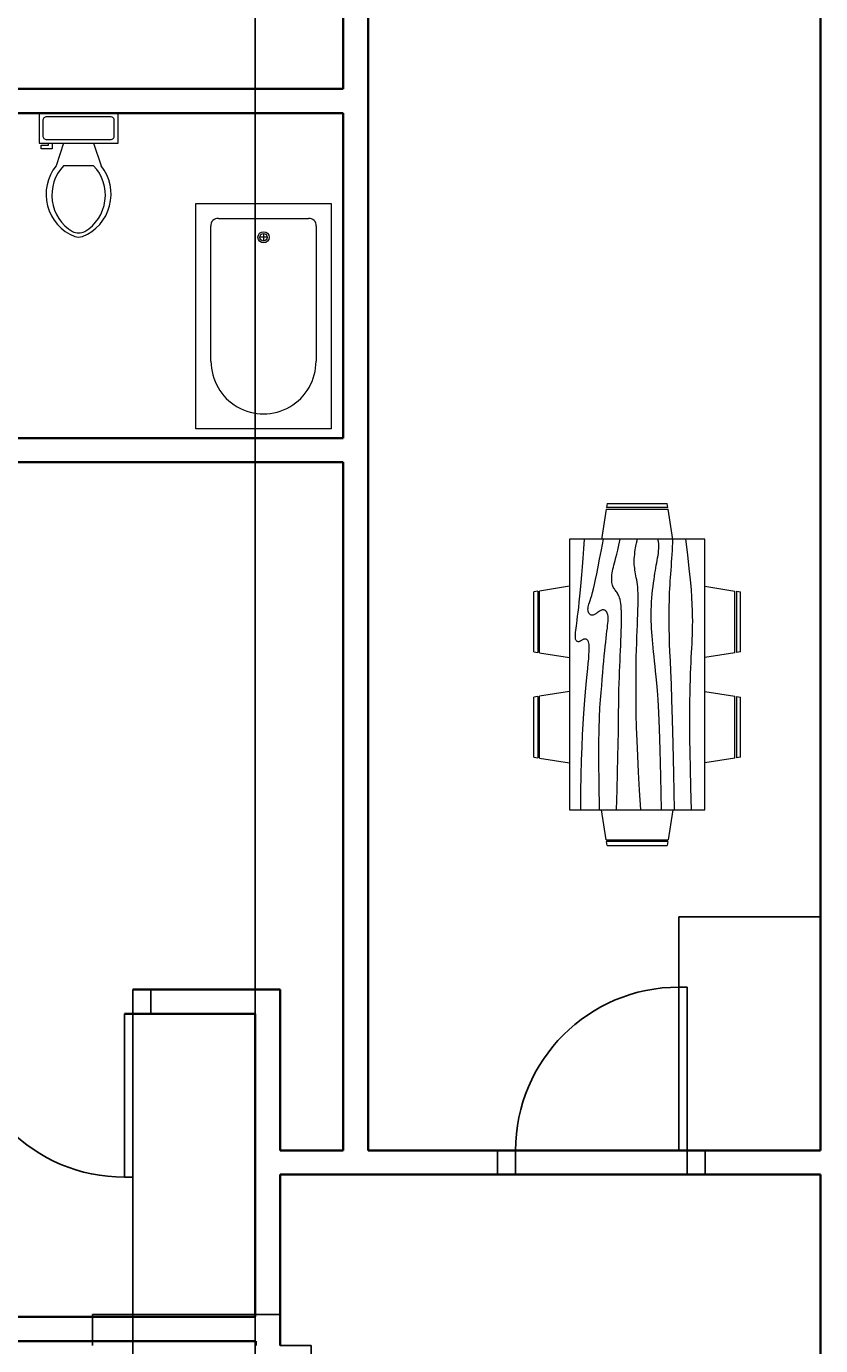
# Model space of a CAD drawing. Units: millimetres. Extents: x 31 to 27050, y -916 to 32407.
# Tile 5 of 7: x 7965 to 13341, y 16782 to 25704. Entities that reach past the tile are written whole.
import ezdxf

# ---------------------------------------------------------------- set-up
doc = ezdxf.new("R2010")
doc.units = ezdxf.units.MM
for name, color, linetype, lineweight in [('A-ANNO-DIMS', 2, 'Continuous', 18), ('A-DOOR', 3, 'Continuous', 25), ('A-FLOR-FIXT', 9, 'Continuous', 18), ('A-FURN', 8, 'Continuous', 13), ('A-WALL', 7, 'Continuous', 35)]:
    doc.layers.add(name, color=color, linetype=linetype, lineweight=lineweight)
doc.styles.get("Standard").update_dxf_attribs({"font": 'arial.ttf'})
doc.dimstyles.get("Standard").update_dxf_attribs({"dimtxt": 0.18, "dimasz": 0.18, "dimexe": 0.18, "dimexo": 0.0625, "dimgap": 0.09, "dimtad": 0, "dimtih": 1, "dimtoh": 1, "dimdec": 4, "dimzin": 0, "dimdsep": 46, "dimtxsty": 'Standard', "dimcen": 0.09, "dimadec": 0, "dimazin": 0, "dimtfac": 1, "dimtdec": 4, "dimtofl": 0, "dimtmove": 0, "dimatfit": 3, "dimfxl": 1, "dimtolj": 1, "dimtzin": 0, "dimarcsym": 0})

# ---------------------------------------------------------------- blocks, each defined once
blk = doc.blocks.new('Dining Set - 36 x 72 in.')
for p, q in [((-22.23430000000002, 26.00059), (-23.48470000000003, 17.99762)), ((-22.23040000000003, 26), (-5.760800000000017, 26)), ((-22, 27.5), (-22.15620000000001, 26.50042)), ((-5.841600000000028, 26.5), (-22.15340000000003, 26.5)), ((-22, 27.5), (-6, 27.5)), ((-5.843700000000012, 26.49966), (-6, 27.5)), ((-4.515199999999992, 17.99762), (-5.765500000000031, 25.99926)), ((5.765699999999981, 26.00059), (4.515299999999967, 17.99762)), ((5.769599999999968, 26), (22.23919999999998, 26)), ((6, 27.5), (5.843799999999987, 26.50042)), ((22.15839999999997, 26.5), (5.846599999999966, 26.5)), ((6, 27.5), (22, 27.5)), ((22.15629999999999, 26.49966), (22, 27.5)), ((23.48480000000001, 17.99762), (22.23449999999997, 25.99926)), ((36, 18), (-36, 18)), ((-36, 18), (-36, -18)), ((36, -18), (36, 18)), ((-45.49999999999999, 8.000000000000004), (-44.50040000000001, 8.156170000000007)), ((-45.49999999999999, 8.000000000000004), (-45.49999999999999, -7.999999999999996)), ((-44.5, -8.15843), (-44.5, 8.153380000000002)), ((-44.00060000000002, 8.234280000000002), (-35.99760000000003, 9.484740000000006)), ((-44, 8.230410000000003), (-44, -8.239149999999999)), ((44.00059999999996, 8.234280000000002), (35.99759999999998, 9.484740000000006)), ((44, 8.230410000000003), (44, -8.239149999999999)), ((44.5, -8.15843), (44.5, 8.153380000000002)), ((45.49999999999999, 8.000000000000004), (44.50049999999999, 8.156170000000007)), ((45.49999999999999, 8.000000000000004), (45.49999999999999, -7.999999999999996)), ((-44.49970000000002, -8.156309999999994), (-45.49999999999999, -7.999999999999996)), ((-35.99760000000003, -9.484759999999998), (-43.9993, -8.234499999999993)), ((35.99759999999998, -9.484759999999998), (43.9993, -8.234499999999993)), ((44.49969999999995, -8.156309999999994), (45.49999999999999, -7.999999999999996)), ((-36, -18), (36, -18)), ((-22.23430000000002, -26.0006), (-23.48470000000003, -17.99762)), ((-4.515199999999992, -17.99762), (-5.765500000000031, -25.99928)), ((5.765699999999981, -26.0006), (4.515299999999967, -17.99762)), ((23.48480000000001, -17.99762), (22.23449999999997, -25.99928)), ((-22.23040000000003, -26), (-5.760800000000017, -26)), ((-22, -27.5), (-22.15620000000001, -26.50044)), ((-5.841600000000028, -26.5), (-22.15340000000003, -26.5)), ((-22, -27.5), (-6, -27.5)), ((-5.843700000000012, -26.49967), (-6, -27.5)), ((5.769599999999968, -26), (22.23919999999998, -26)), ((6, -27.5), (5.843799999999987, -26.50044)), ((22.15839999999997, -26.5), (5.846599999999966, -26.5)), ((6, -27.5), (22, -27.5)), ((22.15629999999999, -26.49967), (22, -27.5))]:
    blk.add_line(p, q)
for points in [[(-36, 15), (-31.17720000000003, 14.97754), (-26.80790000000002, 14.91406), (-22.85380000000003, 14.81543), (-19.27600000000001, 14.6875), (-16.03620000000001, 14.53613), (-13.09570000000002, 14.36718), (-10.41590000000002, 14.18652), (-7.958300000000008, 14), (-5.690400000000011, 13.81315), (-3.603499999999996, 13.63021), (-1.695400000000006, 13.45508), (0.0364999999999896, 13.29166), (1.594499999999982, 13.14388), (2.981099999999969, 13.01562), (4.198800000000005, 12.9108), (5.25, 12.83333), (6.139299999999991, 12.78613), (6.880200000000002, 12.76823), (7.488299999999981, 12.77767), (7.979199999999991, 12.8125), (8.368499999999983, 12.87077), (8.671899999999994, 12.95052), (8.904899999999998, 13.0498), (9.083300000000008, 13.16666), (9.220499999999959, 13.29899000000001), (9.32159999999999, 13.44401), (9.389499999999998, 13.59879), (9.427099999999996, 13.76041), (9.437299999999993, 13.92594), (9.423200000000008, 14.09245), (9.387499999999989, 14.257), (9.333300000000008, 14.41666), (9.263800000000003, 14.56917), (9.183600000000013, 14.71484), (9.097499999999968, 14.85465), (9.010400000000004, 14.98958), (8.92719999999997, 15.12060000000001), (8.852899999999975, 15.2487), (8.79219999999998, 15.37483), (8.75, 15.5), (8.730500000000006, 15.62467), (8.734399999999994, 15.74739), (8.761699999999962, 15.86621), (8.8125, 15.97916), (8.886699999999962, 16.08431), (8.984399999999994, 16.17968), (9.105500000000006, 16.26334), (9.25, 16.33333), (9.418900000000008, 16.38802), (9.617199999999968, 16.42708), (9.850599999999986, 16.45052), (10.125, 16.45833), (10.44630000000001, 16.45052), (10.82029999999997, 16.42708), (11.25290000000001, 16.38802), (11.75, 16.33333), (12.3184, 16.26318), (12.96940000000001, 16.17838), (13.7151, 16.07991), (14.5677, 15.96875), (15.53949999999997, 15.84586), (16.64259999999996, 15.71224), (17.88929999999999, 15.56884), (19.29169999999999, 15.41666), (20.85899999999998, 15.25667), (22.58789999999999, 15.08984), (24.47210000000001, 14.91715), (26.5052, 14.73958), (28.68090000000001, 14.5581), (30.99289999999996, 14.3737), (33.43469999999996, 14.18733), (36, 14)], [(-36, 10), (-28.97660000000002, 10.14274000000001), (-23.17250000000001, 10.20442), (-18.42410000000001, 10.19775), (-14.5677, 10.13541), (-11.43990000000002, 10.03011), (-8.87700000000001, 9.894530000000007), (-6.715399999999988, 9.741370000000005), (-4.791699999999991, 9.58333), (-2.96980000000002, 9.43082), (-1.224600000000009, 9.285150000000005), (0.4414999999999623, 9.14534), (2.02600000000001, 9.010410000000004), (3.526599999999973, 8.879390000000004), (4.940799999999967, 8.751300000000004), (6.265999999999962, 8.625160000000005), (7.5, 8.500000000000004), (8.641099999999994, 8.375490000000003), (9.691399999999987, 8.253900000000005), (10.65379999999999, 8.13818), (11.53120000000001, 8.031250000000004), (12.32669999999996, 7.936030000000005), (13.043, 7.85547), (13.68309999999997, 7.792480000000001), (14.25, 7.750000000000003), (14.74709999999999, 7.730300000000003), (15.17969999999997, 7.733070000000001), (15.55369999999999, 7.757320000000003), (15.875, 7.80208), (16.14940000000001, 7.866370000000006), (16.38279999999997, 7.94922), (16.58109999999999, 8.04964), (16.75, 8.166660000000004), (16.89439999999996, 8.29915), (17.01429999999999, 8.445310000000003), (17.1089, 8.603190000000001), (17.17709999999999, 8.77083), (17.21799999999996, 8.946290000000001), (17.2305, 9.127600000000005), (17.21369999999996, 9.312820000000006), (17.16669999999999, 9.500000000000004), (17.08949999999999, 9.687500000000004), (16.98699999999996, 9.875000000000004), (16.86489999999998, 10.0625), (16.72919999999999, 10.25), (16.5856, 10.4375), (16.44009999999997, 10.625), (16.29849999999999, 10.8125), (16.16669999999999, 11), (16.05000000000001, 11.18733), (15.95179999999999, 11.3737), (15.8752, 11.5581), (15.8229, 11.73958), (15.798, 11.91715), (15.80340000000001, 12.08984), (15.84199999999998, 12.25667), (15.91669999999999, 12.41666), (16.02949999999998, 12.56836), (16.17840000000001, 12.70833), (16.3605, 12.83268), (16.5729, 12.9375), (16.8127, 13.01888000000001), (17.07679999999999, 13.07291), (17.36250000000001, 13.0957), (17.66669999999999, 13.08333), (17.98939999999999, 13.03312), (18.34179999999998, 12.94726), (18.7382, 12.82918), (19.1927, 12.68229), (19.71949999999998, 12.51001), (20.33269999999999, 12.31575), (21.04649999999998, 12.10294), (21.875, 11.875), (22.83569999999997, 11.63354), (23.95900000000001, 11.37304), (25.27859999999999, 11.08618), (26.82819999999998, 10.76562), (28.64139999999998, 10.40405), (30.75200000000001, 9.994140000000005), (33.1936, 9.528560000000002), (36, 9.000000000000004)], [(-36, 5.500000000000003), (-30.71570000000003, 5.334800000000004), (-26.06900000000002, 5.20963), (-21.99459999999999, 5.11767), (-18.42709999999999, 5.05208), (-15.30090000000001, 5.006020000000003), (-12.55080000000004, 4.972650000000005), (-10.1112, 4.945150000000001), (-7.916699999999991, 4.916660000000003), (-5.908999999999991, 4.881670000000003), (-4.058600000000012, 4.839840000000005), (-2.342899999999985, 4.792150000000003), (-0.7395999999999959, 4.73958), (0.7738999999999692, 4.683100000000006), (2.21999999999997, 4.623700000000003), (3.621299999999962, 4.562330000000006), (5, 4.500000000000003), (6.37299999999999, 4.437820000000005), (7.734399999999993, 4.377600000000004), (9.072299999999984, 4.321290000000001), (10.375, 4.27083), (11.63089999999999, 4.228190000000001), (12.8281, 4.195310000000002), (13.95509999999996, 4.17415), (15, 4.166660000000003), (15.95400000000001, 4.174480000000006), (16.81899999999996, 4.197910000000003), (17.6001, 4.236980000000006), (18.30209999999999, 4.291660000000003), (18.92989999999997, 4.361980000000006), (19.48829999999998, 4.447910000000003), (19.98230000000001, 4.549480000000006), (20.41669999999999, 4.666660000000003), (20.79689999999999, 4.798990000000006), (21.1302, 4.944010000000002), (21.42449999999997, 5.098790000000004), (21.6875, 5.260410000000003), (21.92709999999999, 5.42594), (22.15109999999999, 5.592450000000003), (22.36719999999997, 5.757000000000001), (22.58339999999998, 5.916660000000003), (22.80649999999997, 6.068680000000004), (23.04039999999998, 6.210930000000001), (23.28789999999998, 6.341470000000004), (23.5521, 6.45833), (23.83580000000001, 6.559570000000004), (24.142, 6.643230000000006), (24.4735, 6.707350000000001), (24.83339999999998, 6.750000000000003), (25.2235, 6.76969), (25.642, 6.766920000000002), (26.08580000000001, 6.74267), (26.5521, 6.697910000000003), (27.03789999999998, 6.633620000000004), (27.54039999999998, 6.550780000000006), (28.05649999999997, 6.450360000000006), (28.58339999999998, 6.33333), (29.12419999999997, 6.19987), (29.70709999999997, 6.046870000000001), (30.36609999999996, 5.870440000000005), (31.1354, 5.666660000000003), (32.04929999999996, 5.431640000000005), (33.142, 5.161460000000001), (34.44749999999999, 4.852210000000003), (36, 4.500000000000003)], [(-36, -0.9999999999999964), (-30.79150000000004, -0.6590999999999987), (-26.01949999999999, -0.3821599999999954), (-21.65190000000001, -0.1628399999999992), (-17.65629999999999, 0.0052100000000017), (-14.00049999999999, 0.1283300000000018), (-10.65230000000002, 0.2128900000000051), (-7.579600000000027, 0.2652200000000029), (-4.75, 0.2916600000000038), (-2.134000000000014, 0.2979300000000045), (0.2878000000000043, 0.287110000000002), (2.5317, 0.2616300000000002), (4.614599999999995, 0.2239600000000017), (6.552899999999965, 0.1765100000000039), (8.363299999999981, 0.1217400000000062), (10.06229999999999, 0.0620900000000013), (11.66669999999999, 3.6e-15), (13.18989999999996, -0.0620099999999972), (14.63409999999999, -0.1210999999999949), (15.9982, -0.174319999999998), (17.28129999999999, -0.2187499999999964), (18.48230000000001, -0.2514699999999941), (19.6003, -0.2695299999999996), (20.6343, -0.2700199999999988), (21.58339999999999, -0.2499999999999964), (22.44810000000001, -0.2076799999999999), (23.23570000000001, -0.1458399999999962), (23.95490000000001, -0.0683599999999949), (24.6146, 0.0208300000000001), (25.2235, 0.1178400000000046), (25.79039999999998, 0.2187500000000035), (26.32409999999999, 0.3196600000000025), (26.83339999999998, 0.4166600000000038), (27.32650000000001, 0.5061800000000041), (27.80989999999997, 0.5859300000000012), (28.2894, 0.6539700000000046), (28.77089999999999, 0.7083300000000002), (29.26009999999997, 0.7470700000000045), (29.76299999999998, 0.7682300000000062), (30.28550000000001, 0.7698500000000017), (30.83339999999998, 0.7500000000000036), (31.40879999999999, 0.707840000000001), (31.99939999999998, 0.6471300000000006), (32.589, 0.5727500000000028), (33.16149999999999, 0.4895800000000002), (33.70079999999996, 0.402500000000007), (34.19079999999997, 0.3164000000000051), (34.61529999999999, 0.2361600000000017), (34.95839999999998, 0.1666600000000038), (35.20990000000001, 0.1116500000000009), (35.38479999999998, 0.0703100000000028), (35.50399999999996, 0.0406900000000015), (35.58859999999999, 0.0208300000000001), (35.65940000000001, 0.0087900000000012), (35.73769999999996, 0.0026000000000046), (35.8442, 0.0003200000000056), (36, 3.6e-15)], [(-36, -6.499999999999996), (-27.18430000000001, -6.312669999999993), (-20.084, -6.126299999999996), (-14.46899999999999, -5.941899999999993), (-10.10939999999999, -5.760419999999999), (-6.77520000000004, -5.582849999999996), (-4.236300000000028, -5.410159999999994), (-2.262900000000001, -5.243329999999996), (-0.625, -5.083339999999996), (0.8707999999999742, -4.930989999999997), (2.271500000000003, -4.786459999999994), (3.587199999999995, -4.649739999999997), (4.828100000000006, -4.520839999999996), (6.004599999999982, -4.399739999999997), (7.127000000000009, -4.286459999999994), (8.205299999999966, -4.180989999999997), (9.25, -4.083339999999996), (10.27049999999997, -3.993819999999995), (11.27339999999998, -3.914069999999998), (12.2647, -3.846029999999995), (13.25, -3.791669999999999), (14.23539999999997, -3.752929999999995), (15.22659999999996, -3.731769999999993), (16.22949999999997, -3.730149999999998), (17.25, -3.749999999999996), (18.2912, -3.792479999999994), (19.3451, -3.855469999999993), (20.40089999999998, -3.936039999999994), (21.4479, -4.031249999999996), (22.47539999999998, -4.138189999999998), (23.47269999999998, -4.253909999999994), (24.4289, -4.375489999999995), (25.33339999999999, -4.499999999999996), (26.17849999999999, -4.624919999999999), (26.96940000000001, -4.749349999999996), (27.71449999999999, -4.872809999999997), (28.4219, -4.994789999999998), (29.09999999999996, -5.114829999999994), (29.75720000000001, -5.232419999999994), (30.40159999999997, -5.347089999999997), (31.04169999999999, -5.458339999999996), (31.68369999999999, -5.564369999999993), (32.32619999999997, -5.658209999999993), (32.9658, -5.731529999999995), (33.59899999999999, -5.776039999999998), (34.22239999999999, -5.783449999999998), (34.83269999999999, -5.745449999999994), (35.4264, -5.653729999999999), (36, -5.499999999999996)], [(-36, -9.999999999999996), (-26.40219999999999, -9.812989999999996), (-18.46750000000003, -9.628909999999994), (-11.9839, -9.450689999999998), (-6.739599999999995, -9.281249999999996), (-2.522600000000011, -9.123539999999995), (0.8788999999999872, -8.980469999999993), (3.676899999999989, -8.854979999999994), (6.083300000000008, -8.749999999999996), (8.276700000000005, -8.667649999999998), (10.30209999999999, -8.606769999999994), (12.1712, -8.565429999999996), (13.89580000000001, -8.54167), (15.48759999999998, -8.533529999999995), (16.95830000000001, -8.539069999999999), (18.31970000000001, -8.556319999999994), (19.58339999999998, -8.583339999999996), (20.76159999999999, -8.618409999999994), (21.86849999999998, -8.660809999999994), (22.91879999999998, -8.710039999999996), (23.9271, -8.765629999999998), (24.90809999999999, -8.827069999999996), (25.87629999999996, -8.89388), (26.84649999999999, -8.96558), (27.83339999999999, -9.04167), (28.84739999999999, -9.121179999999997), (29.88279999999998, -9.201169999999994), (30.93000000000001, -9.278239999999993), (31.97919999999999, -9.348959999999995), (33.02049999999997, -9.409909999999998), (34.04429999999996, -9.45768), (35.04069999999996, -9.488849999999996), (36, -9.499999999999996)], [(-36, -14.5), (-30.0881, -14.33512999999999), (-25.03320000000002, -14.21224), (-20.7312, -14.12646999999999), (-17.0781, -14.07292), (-13.97000000000003, -14.04670999999999), (-11.30270000000001, -14.04296999999999), (-8.972399999999993, -14.05680999999999), (-6.875, -14.08333999999999), (-4.922400000000038, -14.11832999999999), (-3.09050000000002, -14.16015999999999), (-1.370900000000006, -14.20784999999999), (0.2447999999999979, -14.26042), (1.764700000000004, -14.31689999999999), (3.197299999999984, -14.37629999999999), (4.550700000000006, -14.43766999999999), (5.833300000000008, -14.5), (7.055399999999963, -14.5621), (8.235000000000014, -14.62174999999999), (9.392200000000003, -14.67652), (10.54689999999999, -14.72395999999999), (11.7192, -14.76164), (12.92899999999997, -14.78711), (14.19649999999996, -14.79794), (15.54169999999999, -14.79167), (16.99329999999998, -14.76423999999999), (18.61519999999996, -14.70508), (20.48039999999998, -14.60197), (22.66149999999999, -14.44270999999999), (25.2312, -14.21509), (28.26240000000002, -13.90689999999999), (31.8277, -13.50594), (36, -13)]]:
    blk.add_lwpolyline(points)
blk = doc.blocks.new('Bath Tub - 26 x 60 in.')
for p, q in [((9, -17), (9, -19)), ((8, -18), (10, -18))]:
    blk.add_line(p, q)
blk.add_lwpolyline([(0, -36), (0, 0), (60, 0), (60, -36)], close=True)
for points in [[(4, -30), (4, -6)], [(6, -4), (42, -4)], [(42, -32), (6, -32)]]:
    blk.add_lwpolyline(points)
for radius in [1.5, 1]:
    blk.add_circle((9, -18), radius)
for centre, radius, start, end in [((5.75, -5.75), 1.767766999999999, 81.86989999999999, 188.1301), ((42, -18), 14, 270, 90), ((5.75, -30.25), 1.767766999999999, 171.8699, 278.1301)]:
    blk.add_arc(centre, radius, start, end)
blk = doc.blocks.new('Toilet - top')
for p, q in [((9.5, -6), (9.5, -2)), ((-10, -8.5), (-8, -8.5)), ((-10, -9.5), (-10, -8.5)), ((-7, -9.5), (-10, -9.5)), ((-8, -8.5), (-8, -8)), ((-7, -8), (-7, -9.5)), ((-4, -8), (-6, -14)), ((4, -8), (6, -14)), ((4, -14), (-4, -14))]:
    blk.add_line(p, q)
blk.add_lwpolyline([(10.5, -8), (10.5, 0), (-10.5, 0), (-10.5, -8)], close=True)
for points in [[(-9.5, -2), (-9.5, -6)], [(8.5, -1), (-8.5, -1)], [(-8.5, -7), (8.5, -7)]]:
    blk.add_lwpolyline(points)
for centre, radius, start, end in [((-8.625, -1.875), 0.8838834999999999, 81.86989999999999, 188.1301), ((8.625, -1.875), 0.8838834999999999, 351.8699, 98.13009999999998), ((-8.625, -6.125), 0.8838834999999999, 171.869898, 278.1301), ((8.625, -6.125), 0.8838834999999999, 261.8699, 8.130099999999993), ((3.519562435188956, -21.58049502388982), 12.16902005083646, 141.4691096810948, 247.9714346835576), ((4.199957580658807, -21.81740929088453), 11.3291791325804, 136.3677254423718, 238.946823937405), ((-3.519499936778316, -21.58047137067522), 12.16903423757823, 292.0284332733152, 38.53070636800453), ((-4.199890672038477, -21.81738596564128), 11.32918622148567, 301.0530065773863, 43.63209216694732), ((2.09660981727e-05, -27.87646475467881), 4, 245.7318247449371, 294.2681740488959), ((2.09415214183e-05, -28.99996806116075), 4, 254.8605283244437, 285.1394707718433)]:
    blk.add_arc(centre, radius, start, end)
blk = doc.blocks.new('DOOR-SINGLE-1104')
for p, q in [((56.41678681898429, 1104.337341461596), (-7.18501e-11, 1104.337341461596)), ((-7.18501e-11, 1104.337341461596), (-7.18501e-11, 3.638e-12)), ((56.41678681898429, 7.276e-12), (56.41678681898429, 1104.337341461596)), ((-1226.913698425656, -163.8831223050438), (-1226.913698425656, 3.638e-12)), ((-1104.337341461589, 3.638e-12), (-1226.913698425656, 7.276e-12)), ((-1104.337341461589, 3.638e-12), (-1104.337341461589, -163.8831223050438)), ((-7.18501e-11, 3.638e-12), (56.41678681898429, 7.276e-12)), ((56.41678681898429, -163.8831223050438), (56.41678681898429, 3.638e-12)), ((56.41678681898429, 3.638e-12), (178.9931437830519, 3.638e-12)), ((178.9931437830519, 3.638e-12), (178.9931437830519, -163.8831223050438)), ((-1104.337341461589, -163.8831223050438), (-1226.913698425656, -163.8831223050438)), ((178.9931437830519, -163.8831223050438), (56.41678681898429, -163.8831223050438))]:
    blk.add_line(p, q)
blk.add_arc((0, 3.638e-12), 1104.337341461589, 90, 180)
blk = doc.blocks.new('*D16')
at = {"layer": 'A-ANNO-DIMS', "color": 0, "lineweight": -2, "transparency": 16777216}
for p, q in [((9681.744557342236, 16781.90361905769), (9892.748083673547, 16781.90361905769)), ((9892.568083673546, 16781.72361905769), (9892.568083673546, 16079.13332892196)), ((9892.568083673546, 15376.17677684898), (9892.568083673546, 16078.76706698471)), ((9681.744557342237, 15375.99677684898), (9892.748083673547, 15375.99677684898))]:
    blk.add_line(p, q, dxfattribs=at)
at = {"layer": 'A-ANNO-DIMS', "color": 0, "transparency": 16777216}
for points in [[(9892.538083673546, 16781.72361905769), (9892.598083673547, 16781.72361905769), (9892.568083673546, 16781.90361905769)], [(9892.538083673546, 15376.17677684898), (9892.598083673547, 15376.17677684898), (9892.568083673546, 15375.99677684898)]]:
    blk.add_solid(points, dxfattribs=at)
at = {"layer": 'Defpoints', "color": 0, "transparency": 16777216}
for p in [(9681.682057342236, 16781.90361905769), (9892.568083673546, 16781.90361905769), (9681.682057342237, 15375.99677684898)]:
    blk.add_point(p, dxfattribs=at)
at = {"layer": 'A-ANNO-DIMS', "color": 0, "transparency": 16777216, "insert": (9892.568083673552, 16078.95019795333), "char_height": 0.18, "attachment_point": 5}
blk.add_mtext('\\A1;DOOR 1406 TYP.', dxfattribs=at)
blk = doc.blocks.new('*D17')
at = {"layer": 'A-ANNO-DIMS', "color": 0, "lineweight": -2, "transparency": 16777216}
for p, q in [((8413.461593575592, 16781.96611905768), (8413.461593575592, 16992.96964538898)), ((8413.641593575592, 16992.78964538898), (9046.912357518939, 16992.78964538899)), ((9681.502057342232, 16992.78964538899), (9048.231293398885, 16992.78964538899)), ((9681.682057342232, 16781.96611905768), (9681.682057342232, 16992.96964538899))]:
    blk.add_line(p, q, dxfattribs=at)
at = {"layer": 'A-ANNO-DIMS', "color": 0, "transparency": 16777216}
for points in [[(8413.641593575592, 16992.81964538898), (8413.641593575592, 16992.75964538898), (8413.461593575592, 16992.78964538898)], [(9681.502057342232, 16992.81964538899), (9681.502057342232, 16992.75964538899), (9681.682057342232, 16992.78964538899)]]:
    blk.add_solid(points, dxfattribs=at)
at = {"layer": 'Defpoints', "color": 0, "transparency": 16777216}
for p in [(8413.461593575592, 16992.78964538898), (8413.461593575592, 16781.90361905768), (9681.682057342232, 16781.90361905768)]:
    blk.add_point(p, dxfattribs=at)
at = {"layer": 'A-ANNO-DIMS', "color": 0, "transparency": 16777216, "insert": (9047.571825458914, 16992.78964538899), "char_height": 0.18, "attachment_point": 5}
blk.add_mtext('\\A1;1268 TYP.', dxfattribs=at)
blk = doc.blocks.new('*D66')
at = {"layer": 'A-ANNO-DIMS', "color": 0, "lineweight": -2, "transparency": 16777216}
for p, q in [((2925.691486, 19025.498224), (2925.691486000001, 32406.711259)), ((2925.871486000001, 32406.531259), (6219.151999023875, 32406.531259)), ((9513.151407, 32406.531259), (6219.870893976127, 32406.531259)), ((9513.331407, 19025.498224), (9513.331407, 32406.711259))]:
    blk.add_line(p, q, dxfattribs=at)
at = {"layer": 'A-ANNO-DIMS', "color": 0, "transparency": 16777216}
for points in [[(2925.871486000001, 32406.561259), (2925.871486000001, 32406.501259), (2925.691486000001, 32406.531259)], [(9513.151407, 32406.561259), (9513.151407, 32406.501259), (9513.331407, 32406.531259)]]:
    blk.add_solid(points, dxfattribs=at)
at = {"layer": 'Defpoints', "color": 0, "transparency": 16777216}
for p in [(9513.331407, 32406.531259), (2925.691486, 19025.435724), (9513.331407, 19025.435724)]:
    blk.add_point(p, dxfattribs=at)
at = {"layer": 'A-ANNO-DIMS', "color": 0, "transparency": 16777216, "insert": (6219.511446500001, 32406.531259), "char_height": 0.18, "attachment_point": 5}
blk.add_mtext('\\A1;6588', dxfattribs=at)
blk = doc.blocks.new('*D73')
at = {"layer": 'A-ANNO-DIMS', "color": 0, "lineweight": -2, "transparency": 16777216}
for p, q in [((12380.499727, 18102.073129), (12380.499727, 19681.190629)), ((12380.679727, 19681.010629), (12860.25398975443, 19681.010629)), ((13340.405333, 19681.010629), (12860.83107024557, 19681.010629)), ((13340.585333, 18102.073129), (13340.585333, 19681.190629))]:
    blk.add_line(p, q, dxfattribs=at)
at = {"layer": 'A-ANNO-DIMS', "color": 0, "transparency": 16777216}
for points in [[(12380.679727, 19681.040629), (12380.679727, 19680.980629), (12380.499727, 19681.010629)], [(13340.405333, 19681.040629), (13340.405333, 19680.980629), (13340.585333, 19681.010629)]]:
    blk.add_solid(points, dxfattribs=at)
at = {"layer": 'Defpoints', "color": 0, "transparency": 16777216}
for p in [(13340.585333, 19681.010629), (12380.499727, 18102.010629), (13340.585333, 18102.010629)]:
    blk.add_point(p, dxfattribs=at)
at = {"layer": 'A-ANNO-DIMS', "color": 0, "transparency": 16777216, "insert": (12860.54253, 19681.010629), "char_height": 0.18, "attachment_point": 5}
blk.add_mtext('\\A1;960', dxfattribs=at)
blk = doc.blocks.new('*D74')
at = {"layer": 'A-ANNO-DIMS', "color": 0, "lineweight": -2, "transparency": 16777216}
for p, q in [((8684.522829, 19025.373224), (8684.522828999998, -915.5318640000004)), ((9513.331407, 19025.373224), (9513.331407, -915.5318640000004)), ((8684.702829, -915.3518639999999), (9098.533107085947, -915.3518639999999)), ((9513.151406999998, -915.3518639999999), (9099.321128914047, -915.3518639999999))]:
    blk.add_line(p, q, dxfattribs=at)
at = {"layer": 'A-ANNO-DIMS', "color": 0, "transparency": 16777216}
for points in [[(8684.702829, -915.321864), (8684.702829, -915.381864), (8684.522828999998, -915.3518639999999)], [(9513.151406999998, -915.321864), (9513.151406999998, -915.381864), (9513.331407, -915.3518639999999)]]:
    blk.add_solid(points, dxfattribs=at)
at = {"layer": 'Defpoints', "color": 0, "transparency": 16777216}
for p in [(8684.522829, 19025.435724), (9513.331407, 19025.435724), (8684.522828999998, -915.3518639999999)]:
    blk.add_point(p, dxfattribs=at)
at = {"layer": 'A-ANNO-DIMS', "color": 0, "transparency": 16777216, "insert": (9098.927117999998, -915.3518639999999), "char_height": 0.18, "attachment_point": 5}
blk.add_mtext('\\A1;828.8', dxfattribs=at)

msp = doc.modelspace()

# ---------------------------------------------------------------- linework, layer by layer
at = {"layer": 'A-WALL'}
for p, q in [((10110.02199711446, 25282.64192458121), (10110.02199711446, 30663.64813636668)), ((10278.37264782516, 24473.25786145121), (10278.37264782516, 29309.37473914616)), ((13340.58533261045, 29309.37473914617), (13340.58533261045, 24473.25786145121)), ((6778.372647825161, 25282.64192458121), (10110.02199711446, 25282.64192458121)), ((10110.02199711446, 25117.33256545015), (6778.372647825162, 25117.33256545015)), ((10110.02199711446, 22919.96829640664), (10110.02199711446, 25117.33256545015)), ((10278.37264782516, 24473.25786145121), (10278.37264782516, 24309.37473914615)), ((13340.58533261045, 24473.25786145121), (13340.58533261045, 24309.37473914616)), ((10278.37264782516, 18469.90100734673), (10278.37264782516, 24309.37473914615)), ((13340.58533261045, 18102.01062910059), (13340.58533261045, 24309.37473914616)), ((6778.372647825161, 22919.96829640664), (10110.02199711446, 22919.96829640664)), ((6690.585332610448, 22756.08517410159), (10110.02199711446, 22756.08517410159)), ((10110.02199711446, 18469.90100734673), (10110.02199711446, 22756.08517410159)), ((9593.894742127508, 19189.3188461972), (8684.522828904213, 19189.31884619719)), ((9681.68205734222, 19189.3188461972), (9544.65935867536, 19189.3188461972)), ((9681.68205734222, 18895.47530332579), (9681.68205734222, 19189.3188461972)), ((9513.331406631527, 19025.43572389214), (8628.106042085157, 19025.43572389214)), ((9513.331406631525, 18895.47530332579), (9513.331406631527, 19025.43572389215)), ((9513.331406631527, 16976.9449186614), (9513.331406631525, 18895.47530332579)), ((9681.68205734222, 18102.0106291006), (9681.68205734222, 18895.47530332579)), ((10110.02199711446, 18469.90100734673), (10110.02199711446, 18102.0106291006)), ((10278.37264782516, 18469.90100734673), (10278.37264782516, 18102.0106291006)), ((9681.682057342217, 18102.0106291006), (10110.02199711446, 18102.0106291006)), ((10278.37264782516, 18102.0106291006), (13340.58533261045, 18102.01062910059)), ((9681.682057342221, 17938.12750679554), (13340.58533261045, 17938.12750679554)), ((9681.682057342221, 16893.79403776525), (9681.682057342221, 17938.12750679554)), ((13340.58533261045, 13102.01062910059), (13340.58533261045, 17938.12750679554)), ((2925.691486399058, 16976.94491866139), (9513.331406631527, 16976.9449186614)), ((9681.682057342221, 16893.79403776525), (9681.682057342221, 16813.06179635634)), ((2757.340835688364, 16813.06179635634), (9517.798935037174, 16813.06179635634)), ((9517.798935037174, 16781.90361905769), (9517.798935037174, 16813.06179635634)), ((9681.682057342221, 16813.06179635634), (9681.682057342221, 16781.90361905769))]:
    msp.add_line(p, q, dxfattribs=at)

# ---------------------------------------------------------------- block references
at = {"layer": 'A-DOOR', "extrusion": (0, 0, -1), "zscale": -1, "rotation": 180}
msp.add_blockref('DOOR-SINGLE-1104', (-8628.10604208523, 19025.43572389217), dxfattribs=at)
at = {"layer": 'A-DOOR'}
msp.add_blockref('DOOR-SINGLE-1104', (12380.49972657995, 18102.01062910057), dxfattribs=at)
at = {"layer": 'A-FLOR-FIXT', "xscale": 25.4, "yscale": 25.4, "zscale": 25.4}
msp.add_blockref('Toilet - top', (8318.536898579667, 25117.33256545015), dxfattribs=at)
at = {"layer": 'A-FLOR-FIXT', "xscale": 25.4, "yscale": 25.4, "zscale": 25.4, "rotation": 270}
msp.add_blockref('Bath Tub - 26 x 60 in.', (10027.33293622188, 24506.11473923286), dxfattribs=at)
at = {"layer": 'A-FURN', "xscale": 25.4, "yscale": 25.4, "zscale": 25.4, "rotation": 90}
msp.add_blockref('Dining Set - 36 x 72 in.', (12098.65736106344, 21320.51173650057), dxfattribs=at)

# ---------------------------------------------------------------- dimensions: what is measured, and where the dimension line sits
at = {"layer": 'A-ANNO-DIMS'}
for base, p1, p2, override, picture, middle in [((9513.331407, 32406.531259), (2925.691486, 19025.435724), (9513.331407, 19025.435724), {"dimdec": 0, "dimlfac": 1, "dimrnd": 0, "dimzin": 0, "dimdsep": 46, "dimlunit": 2}, '*D66', (6219.511446500001, 32406.531259)), ((8684.522828999998, -915.3518639999999), (9513.331407, 19025.435724), (8684.522829, 19025.435724), {"dimdec": 1, "dimlfac": 1, "dimrnd": 0, "dimzin": 0, "dimdsep": 46, "dimlunit": 2}, '*D74', (9098.927117999998, -915.3518639999999))]:
    dim = msp.add_linear_dim(base=base, p1=p1, p2=p2, dimstyle='Standard', override=override, dxfattribs=at)
    dim.commit()
    dim.dimension.update_dxf_attribs({"geometry": picture, "text_midpoint": middle})
dim = msp.add_linear_dim(base=(13340.585333, 19681.010629), p1=(12380.499727, 18102.010629), p2=(13340.585333, 18102.010629), angle=1.0855e-12, dimstyle='Standard', override={"dimdec": 0, "dimlfac": 1, "dimrnd": 0, "dimzin": 0, "dimdsep": 46, "dimlunit": 2}, dxfattribs=at)
dim.commit()
dim.dimension.update_dxf_attribs({"geometry": '*D73', "text_midpoint": (12860.54253, 19681.010629)})
for base, p1, p2, angle, text, picture, middle in [((8413.461593575592, 16992.78964538898), (9681.682057342232, 16781.90361905768), (8413.461593575592, 16781.90361905768), 180.0000000000001, '<> TYP.', '*D17', (9047.571825458914, 16992.78964538899)), ((9892.568083673546, 16781.90361905769), (9681.682057342234, 15375.99677684897), (9681.682057342232, 16781.90361905768), 90.00000000000007, 'DOOR <> TYP.', '*D16', (9892.568083673552, 16078.95019795333))]:
    dim = msp.add_linear_dim(base=base, p1=p1, p2=p2, angle=angle, text=text, dimstyle='Standard', override={"dimdec": 0, "dimlfac": 1, "dimrnd": 0, "dimzin": 0, "dimdsep": 46, "dimlunit": 2}, dxfattribs=at)
    dim.commit()
    dim.dimension.update_dxf_attribs({"geometry": picture, "text_midpoint": middle})

doc.saveas('drawing.dxf')
